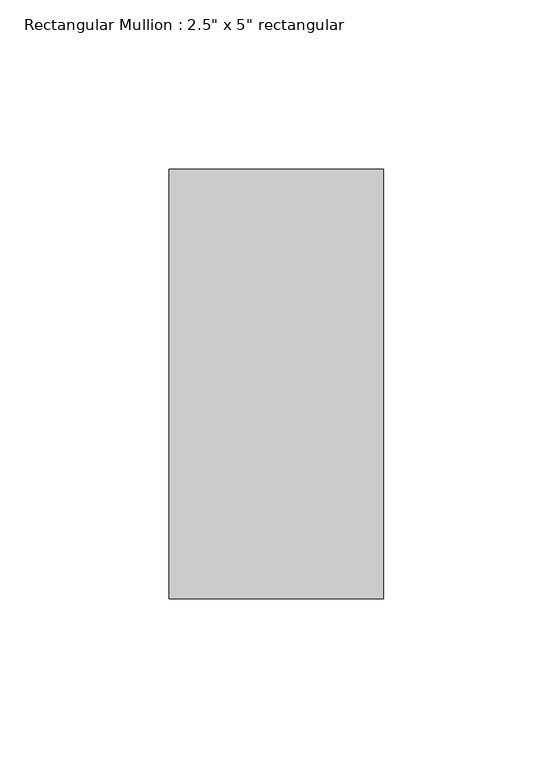
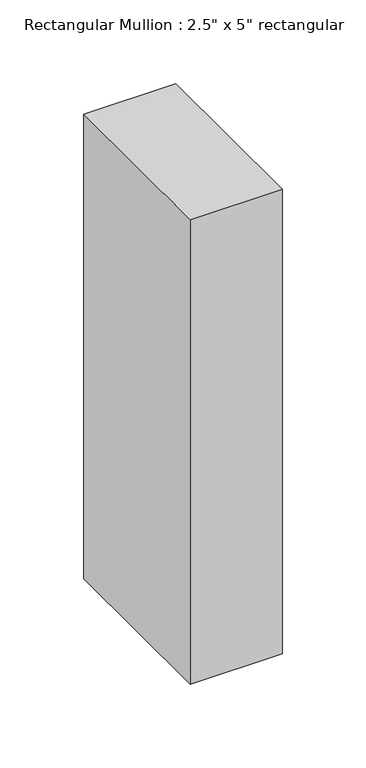
"""IFC4 building model written with IfcOpenShell, lengths in millimetres: member geometry."""

from ifc_helpers import new_model, si_unit, frame, origin, place, context, project, spatial, polyline, outline, extrude, source, transform, mapped, element, save


def member_b2812fca(model_context):
    return source(origin(), model_context, "Body", "SweptSolid", [
        extrude(outline(polyline([(31.75, 63.5), (31.75, -63.5), (-31.75, -63.5), (-31.75, 63.5), (31.75, 63.5)])), frame((0.0, 0.0, -338.6666667), z_axis=(0.0, 0.0, 1.0), x_axis=(1.0, 0.0, 0.0)), (0.0, 0.0, 1.0), 338.6666667),
    ])


if __name__ == "__main__":
    model = new_model("IFC4")
    model_context = context("Model", 3, world=origin())
    ifc_project = project(units=[si_unit("LENGTHUNIT", "METRE", prefix="MILLI")], contexts=[model_context])
    site = spatial("IfcSite", under=ifc_project)
    building = spatial("IfcBuilding", under=site)
    placement = place(None, origin())
    member_shape = member_b2812fca(model_context)
    element("IfcMember", 1, ObjectType="Rectangular Mullion : 2.5\" x 5\" rectangular", at=placement, inside=building, context=model_context, shape_type="MappedRepresentation", body=[
        mapped(member_shape, transform((0.0, 0.0, 0.0), x_axis=(1.0, 0.0, 0.0), y_axis=(0.0, 1.0, 0.0), z_axis=(0.0, 0.0, 1.0))),
    ])
    save(model, "model.ifc")

# Revit data of these elements
# Type "Rectangular Mullion : 2.5\" x 5\" rectangular"
#   built-in parameter 1007304 = 0.416667 (stored number, unit not read)
#   built-in parameter 1007301 = 0.104167 (stored number, unit not read)
#   built-in parameter 1007300 = 0.104167 (stored number, unit not read)
# Element 1 (IfcMember, "Rectangular Mullion : 2.5\" x 5\" rectangular")
#   Materials on its faces: "door colour"
# Materials
#   "door colour": class "Generic", colour RGB 120 120 120, transparency 0, Cost = 0
